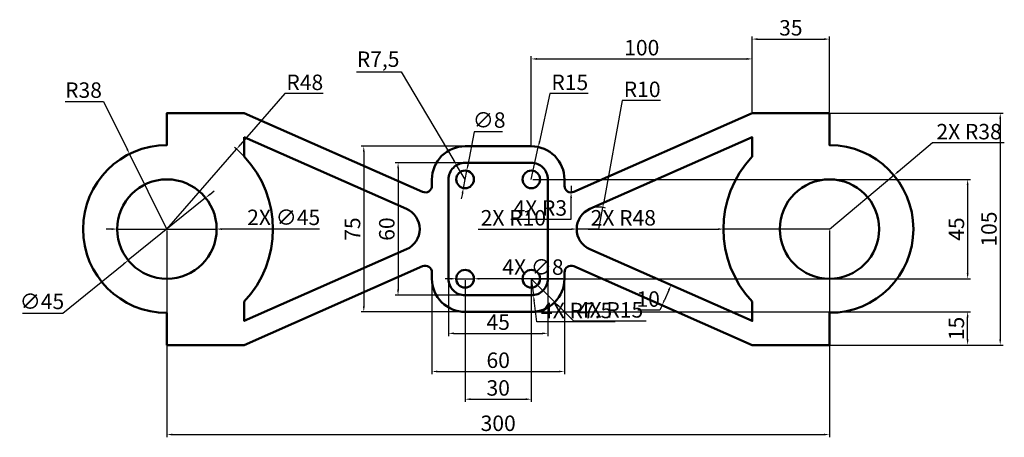
# Model space of a CAD drawing. Units: millimetres. Extents: x 172 to 618, y 203 to 392.
import ezdxf

# ---------------------------------------------------------------- set-up
doc = ezdxf.new("R2010")
doc.units = ezdxf.units.MM
doc.layers.add('M-DIMS', color=2, linetype='Continuous', lineweight=25)
doc.layers.add('M-OUTL', color=7, linetype='Continuous', lineweight=50)
doc.styles.get("Standard").update_dxf_attribs({"font": 'arial.ttf'})
doc.dimstyles.new('ISO-25', dxfattribs={"dimtxt": 7, "dimasz": 2.5, "dimexe": 1.25, "dimexo": 0.625, "dimtad": 1, "dimtoh": 1, "dimtxsty": 'Standard', "dimcen": 2.5, "dimadec": 0, "dimazin": 0, "dimtfac": 1, "dimtmove": 0, "dimatfit": 3, "dimfxl": 1, "dimarcsym": 0})

# ---------------------------------------------------------------- blocks, each defined once
blk = doc.blocks.new('*D1')
at = {"layer": 'Defpoints', "color": 0, "transparency": 16777216}
for p in [(370.22, 326.21), (374.05, 319.76)]:
    blk.add_point(p, dxfattribs=at)
at = {"layer": 'M-DIMS', "color": 0, "lineweight": -2, "transparency": 16777216}
for p, q in [((324.93, 368.48), (345.06, 368.48)), ((345.06, 368.48), (368.94, 328.35)), ((374.05, 319.76), (370.22, 326.21))]:
    blk.add_line(p, q, dxfattribs=at)
at = {"layer": 'M-DIMS', "color": 0, "transparency": 16777216}
blk.add_solid([(369.3, 328.57), (368.58, 328.14), (370.22, 326.21)], dxfattribs=at)
at = {"layer": 'M-DIMS', "color": 0, "transparency": 16777216, "insert": (334.68, 373.3), "char_height": 7, "attachment_point": 5}
blk.add_mtext('R7,5', dxfattribs=at)
blk = doc.blocks.new('*D2')
at = {"layer": 'Defpoints', "color": 0, "transparency": 16777216}
for p in [(407.22, 334.42), (404.05, 319.76)]:
    blk.add_point(p, dxfattribs=at)
at = {"layer": 'M-DIMS', "color": 0, "lineweight": -2, "transparency": 16777216}
for p, q in [((412.44, 358.61), (407.75, 336.87)), ((429.85, 358.61), (412.44, 358.61)), ((404.05, 319.76), (407.22, 334.42))]:
    blk.add_line(p, q, dxfattribs=at)
at = {"layer": 'M-DIMS', "color": 0, "transparency": 16777216}
blk.add_solid([(407.34, 336.96), (408.15, 336.78), (407.22, 334.42)], dxfattribs=at)
at = {"layer": 'M-DIMS', "color": 0, "transparency": 16777216, "insert": (421.46, 362.81), "char_height": 7, "attachment_point": 5}
blk.add_mtext('R15', dxfattribs=at)
blk = doc.blocks.new('*D3')
at = {"layer": 'Defpoints', "color": 0, "transparency": 16777216}
for p in [(389.05, 334.76), (328.19, 259.76), (389.05, 259.76)]:
    blk.add_point(p, dxfattribs=at)
at = {"layer": 'M-DIMS', "color": 0, "lineweight": -2, "transparency": 16777216}
for p, q in [((388.43, 334.76), (326.94, 334.76)), ((328.19, 332.26), (328.19, 262.26)), ((388.43, 259.76), (326.94, 259.76))]:
    blk.add_line(p, q, dxfattribs=at)
at = {"layer": 'M-DIMS', "color": 0, "transparency": 16777216}
for points in [[(327.78, 332.26), (328.61, 332.26), (328.19, 334.76)], [(327.78, 262.26), (328.61, 262.26), (328.19, 259.76)]]:
    blk.add_solid(points, dxfattribs=at)
at = {"layer": 'M-DIMS', "color": 0, "transparency": 16777216, "insert": (324.01, 297.26), "char_height": 7, "attachment_point": 5, "rotation": 90}
blk.add_mtext('75', dxfattribs=at)
blk = doc.blocks.new('*D4')
at = {"layer": 'Defpoints', "color": 0, "transparency": 16777216}
for p in [(389.05, 327.26), (343.71, 267.26), (389.05, 267.26)]:
    blk.add_point(p, dxfattribs=at)
at = {"layer": 'M-DIMS', "color": 0, "lineweight": -2, "transparency": 16777216}
for p, q in [((388.43, 327.26), (342.46, 327.26)), ((343.71, 324.76), (343.71, 269.76)), ((388.43, 267.26), (342.46, 267.26))]:
    blk.add_line(p, q, dxfattribs=at)
at = {"layer": 'M-DIMS', "color": 0, "transparency": 16777216}
for points in [[(343.3, 324.76), (344.13, 324.76), (343.71, 327.26)], [(343.3, 269.76), (344.13, 269.76), (343.71, 267.26)]]:
    blk.add_solid(points, dxfattribs=at)
at = {"layer": 'M-DIMS', "color": 0, "transparency": 16777216, "insert": (339.51, 297.26), "char_height": 7, "attachment_point": 5, "rotation": 90}
blk.add_mtext('60', dxfattribs=at)
blk = doc.blocks.new('*D5')
at = {"layer": 'Defpoints', "color": 0, "transparency": 16777216}
for p in [(270.58, 333.46), (239.05, 297.26)]:
    blk.add_point(p, dxfattribs=at)
at = {"layer": 'M-DIMS', "color": 0, "lineweight": -2, "transparency": 16777216}
for p, q in [((292.49, 358.61), (272.22, 335.34)), ((309.85, 358.61), (292.49, 358.61)), ((239.05, 297.26), (270.58, 333.46))]:
    blk.add_line(p, q, dxfattribs=at)
blk.add_arc((239.05, 297.26), 48, 43.9295, 50.4389, dxfattribs=at)
at = {"layer": 'M-DIMS', "color": 0, "transparency": 16777216}
blk.add_solid([(271.91, 335.62), (272.53, 335.07), (270.58, 333.46)], dxfattribs=at)
at = {"layer": 'M-DIMS', "color": 0, "transparency": 16777216, "insert": (301.48, 362.81), "char_height": 7, "attachment_point": 5}
blk.add_mtext('R48', dxfattribs=at)
blk = doc.blocks.new('*D6')
at = {"layer": 'Defpoints', "color": 0, "transparency": 16777216}
for p in [(222.13, 331.28), (239.05, 297.26)]:
    blk.add_point(p, dxfattribs=at)
at = {"layer": 'M-DIMS', "color": 0, "lineweight": -2, "transparency": 16777216}
for p, q in [((192.92, 355.09), (210.28, 355.09)), ((210.28, 355.09), (221.01, 333.52)), ((239.05, 297.26), (222.13, 331.28))]:
    blk.add_line(p, q, dxfattribs=at)
at = {"layer": 'M-DIMS', "color": 0, "transparency": 16777216}
blk.add_solid([(221.39, 333.71), (220.64, 333.34), (222.13, 331.28)], dxfattribs=at)
at = {"layer": 'M-DIMS', "color": 0, "transparency": 16777216, "insert": (201.29, 359.29), "char_height": 7, "attachment_point": 5}
blk.add_mtext('R38', dxfattribs=at)
blk = doc.blocks.new('*D7')
at = {"layer": 'Defpoints', "color": 0, "transparency": 16777216}
for p in [(256.56, 311.4), (221.55, 283.12)]:
    blk.add_point(p, dxfattribs=at)
at = {"layer": 'M-DIMS', "color": 0, "lineweight": -2, "transparency": 16777216}
for p, q in [((258.5, 312.97), (260.45, 314.54)), ((256.56, 311.4), (221.55, 283.12)), ((191.94, 259.2), (219.61, 281.55)), ((173.61, 259.2), (191.94, 259.2))]:
    blk.add_line(p, q, dxfattribs=at)
at = {"layer": 'M-DIMS', "color": 0, "transparency": 16777216}
for points in [[(258.24, 313.29), (258.76, 312.65), (256.56, 311.4)], [(219.34, 281.88), (219.87, 281.23), (221.55, 283.12)]]:
    blk.add_solid(points, dxfattribs=at)
at = {"layer": 'M-DIMS', "color": 0, "transparency": 16777216, "insert": (182.46, 263.6), "char_height": 7, "attachment_point": 5}
blk.add_mtext('∅45', dxfattribs=at)
blk = doc.blocks.new('*D8')
at = {"layer": 'Defpoints', "color": 0, "transparency": 16777216}
for p in [(239.05, 297.26), (539.05, 297.26), (539.05, 204.21)]:
    blk.add_point(p, dxfattribs=at)
at = {"layer": 'M-DIMS', "color": 0, "lineweight": -2, "transparency": 16777216}
for p, q in [((239.05, 296.64), (239.05, 202.96)), ((539.05, 296.64), (539.05, 202.96)), ((241.55, 204.21), (536.55, 204.21))]:
    blk.add_line(p, q, dxfattribs=at)
at = {"layer": 'M-DIMS', "color": 0, "transparency": 16777216}
for points in [[(241.55, 204.62), (241.55, 203.79), (239.05, 204.21)], [(536.55, 204.62), (536.55, 203.79), (539.05, 204.21)]]:
    blk.add_solid(points, dxfattribs=at)
at = {"layer": 'M-DIMS', "color": 0, "transparency": 16777216, "insert": (389.05, 208.41), "char_height": 7, "attachment_point": 5}
blk.add_mtext('300', dxfattribs=at)
blk = doc.blocks.new('*D9')
at = {"layer": 'Defpoints', "color": 0, "transparency": 16777216}
for p in [(359.05, 274.76), (419.05, 274.76), (419.05, 232.76)]:
    blk.add_point(p, dxfattribs=at)
at = {"layer": 'M-DIMS', "color": 0, "lineweight": -2, "transparency": 16777216}
for p, q in [((359.05, 274.14), (359.05, 231.51)), ((419.05, 274.14), (419.05, 231.51)), ((361.55, 232.76), (416.55, 232.76))]:
    blk.add_line(p, q, dxfattribs=at)
at = {"layer": 'M-DIMS', "color": 0, "transparency": 16777216}
for points in [[(361.55, 233.18), (361.55, 232.35), (359.05, 232.76)], [(416.55, 233.18), (416.55, 232.35), (419.05, 232.76)]]:
    blk.add_solid(points, dxfattribs=at)
at = {"layer": 'M-DIMS', "color": 0, "transparency": 16777216, "insert": (389.05, 236.96), "char_height": 7, "attachment_point": 5}
blk.add_mtext('60', dxfattribs=at)
blk = doc.blocks.new('*D10')
at = {"layer": 'Defpoints', "color": 0, "transparency": 16777216}
for p in [(366.55, 288.46), (411.55, 288.46), (411.55, 250.04)]:
    blk.add_point(p, dxfattribs=at)
at = {"layer": 'M-DIMS', "color": 0, "lineweight": -2, "transparency": 16777216}
for p, q in [((366.55, 287.84), (366.55, 248.79)), ((411.55, 287.84), (411.55, 248.79)), ((369.05, 250.04), (409.05, 250.04))]:
    blk.add_line(p, q, dxfattribs=at)
at = {"layer": 'M-DIMS', "color": 0, "transparency": 16777216}
for points in [[(369.05, 250.45), (369.05, 249.62), (366.55, 250.04)], [(409.05, 250.45), (409.05, 249.62), (411.55, 250.04)]]:
    blk.add_solid(points, dxfattribs=at)
at = {"layer": 'M-DIMS', "color": 0, "transparency": 16777216, "insert": (389.05, 254.22), "char_height": 7, "attachment_point": 5}
blk.add_mtext('45', dxfattribs=at)
blk = doc.blocks.new('*D11')
at = {"layer": 'Defpoints', "color": 0, "transparency": 16777216}
for p in [(374.81, 323.69), (373.3, 315.83)]:
    blk.add_point(p, dxfattribs=at)
at = {"layer": 'M-DIMS', "color": 0, "lineweight": -2, "transparency": 16777216}
for p, q in [((378.22, 341.34), (375.29, 326.14)), ((391.06, 341.34), (378.22, 341.34)), ((373.3, 315.83), (374.81, 323.69)), ((372.82, 313.38), (372.35, 310.92))]:
    blk.add_line(p, q, dxfattribs=at)
at = {"layer": 'M-DIMS', "color": 0, "transparency": 16777216}
for points in [[(374.88, 326.22), (375.7, 326.06), (374.81, 323.69)], [(372.41, 313.46), (373.23, 313.3), (373.3, 315.83)]]:
    blk.add_solid(points, dxfattribs=at)
at = {"layer": 'M-DIMS', "color": 0, "transparency": 16777216, "insert": (384.95, 345.73), "char_height": 7, "attachment_point": 5}
blk.add_mtext('∅8', dxfattribs=at)
blk = doc.blocks.new('*D12')
at = {"layer": 'Defpoints', "color": 0, "transparency": 16777216}
for p in [(436.4, 307.1), (434.6, 297.26)]:
    blk.add_point(p, dxfattribs=at)
at = {"layer": 'M-DIMS', "color": 0, "lineweight": -2, "transparency": 16777216}
for p, q in [((445.25, 355.44), (436.85, 309.56)), ((462.58, 355.44), (445.25, 355.44)), ((434.6, 297.26), (436.4, 307.1))]:
    blk.add_line(p, q, dxfattribs=at)
blk.add_arc((434.6, 297.26), 10, 72.4639, 110.225, dxfattribs=at)
at = {"layer": 'M-DIMS', "color": 0, "transparency": 16777216}
blk.add_solid([(436.44, 309.63), (437.26, 309.48), (436.4, 307.1)], dxfattribs=at)
at = {"layer": 'M-DIMS', "color": 0, "transparency": 16777216, "insert": (454.23, 359.64), "char_height": 7, "attachment_point": 5}
blk.add_mtext('R10', dxfattribs=at)
blk = doc.blocks.new('*D13')
at = {"layer": 'Defpoints', "color": 0, "transparency": 16777216}
for p in [(539.05, 383.29), (504.05, 349.76), (539.05, 349.76)]:
    blk.add_point(p, dxfattribs=at)
at = {"layer": 'M-DIMS', "color": 0, "lineweight": -2, "transparency": 16777216}
for p, q in [((504.05, 350.39), (504.05, 384.54)), ((539.05, 350.39), (539.05, 384.54)), ((506.55, 383.29), (536.55, 383.29))]:
    blk.add_line(p, q, dxfattribs=at)
at = {"layer": 'M-DIMS', "color": 0, "transparency": 16777216}
for points in [[(506.55, 383.71), (506.55, 382.87), (504.05, 383.29)], [(536.55, 383.71), (536.55, 382.87), (539.05, 383.29)]]:
    blk.add_solid(points, dxfattribs=at)
at = {"layer": 'M-DIMS', "color": 0, "transparency": 16777216, "insert": (521.55, 387.49), "char_height": 7, "attachment_point": 5}
blk.add_mtext('35', dxfattribs=at)
blk = doc.blocks.new('*D14')
at = {"layer": 'Defpoints', "color": 0, "transparency": 16777216}
for p in [(521.55, 349.76), (521.55, 244.76), (616.37, 244.76)]:
    blk.add_point(p, dxfattribs=at)
at = {"layer": 'M-DIMS', "color": 0, "lineweight": -2, "transparency": 16777216}
for p, q in [((522.18, 349.76), (617.62, 349.76)), ((616.37, 347.26), (616.37, 247.26)), ((522.18, 244.76), (617.62, 244.76))]:
    blk.add_line(p, q, dxfattribs=at)
at = {"layer": 'M-DIMS', "color": 0, "transparency": 16777216}
for points in [[(615.95, 347.26), (616.78, 347.26), (616.37, 349.76)], [(615.95, 247.26), (616.78, 247.26), (616.37, 244.76)]]:
    blk.add_solid(points, dxfattribs=at)
at = {"layer": 'M-DIMS', "color": 0, "transparency": 16777216, "insert": (612.17, 297.26), "char_height": 7, "attachment_point": 5, "rotation": 90}
blk.add_mtext('105', dxfattribs=at)
blk = doc.blocks.new('*D15')
at = {"layer": 'Defpoints', "color": 0, "transparency": 16777216}
for p in [(467.31, 271.9), (463.27, 262.75), (463.27, 262.75)]:
    blk.add_point(p, dxfattribs=at)
at = {"layer": 'M-DIMS', "color": 0, "lineweight": -2, "transparency": 16777216}
for p, q in [((466.74, 272.15), (466.17, 272.41)), ((466.3, 269.61), (464.28, 265.04)), ((462.7, 263), (462.13, 263.26)), ((462.26, 260.47), (452.3, 260.47)), ((463.27, 262.75), (462.26, 260.47))]:
    blk.add_line(p, q, dxfattribs=at)
at = {"layer": 'M-DIMS', "color": 0, "transparency": 16777216}
for points in [[(465.92, 269.78), (466.68, 269.45), (467.31, 271.9)], [(463.9, 265.21), (464.66, 264.87), (463.27, 262.75)]]:
    blk.add_solid(points, dxfattribs=at)
at = {"layer": 'M-DIMS', "color": 0, "transparency": 16777216, "insert": (456.97, 264.66), "char_height": 7, "attachment_point": 5}
blk.add_mtext('10', dxfattribs=at)
blk = doc.blocks.new('*D16')
at = {"layer": 'Defpoints', "color": 0, "transparency": 16777216}
for p in [(504.05, 374.31), (504.05, 349.76), (404.05, 334.76)]:
    blk.add_point(p, dxfattribs=at)
at = {"layer": 'M-DIMS', "color": 0, "lineweight": -2, "transparency": 16777216}
for p, q in [((404.05, 335.39), (404.05, 375.56)), ((504.05, 350.39), (504.05, 375.56)), ((406.55, 374.31), (501.55, 374.31))]:
    blk.add_line(p, q, dxfattribs=at)
at = {"layer": 'M-DIMS', "color": 0, "transparency": 16777216}
for points in [[(406.55, 374.73), (406.55, 373.89), (404.05, 374.31)], [(501.55, 374.73), (501.55, 373.89), (504.05, 374.31)]]:
    blk.add_solid(points, dxfattribs=at)
at = {"layer": 'M-DIMS', "color": 0, "transparency": 16777216, "insert": (454.05, 378.51), "char_height": 7, "attachment_point": 5}
blk.add_mtext('100', dxfattribs=at)
blk = doc.blocks.new('*D17')
at = {"layer": 'Defpoints', "color": 0, "transparency": 16777216}
for p in [(404.05, 259.76), (601.6, 259.76), (504.05, 244.76)]:
    blk.add_point(p, dxfattribs=at)
at = {"layer": 'M-DIMS', "color": 0, "lineweight": -2, "transparency": 16777216}
for p, q in [((404.68, 259.76), (602.85, 259.76)), ((601.6, 247.26), (601.6, 257.26)), ((504.68, 244.76), (602.85, 244.76))]:
    blk.add_line(p, q, dxfattribs=at)
at = {"layer": 'M-DIMS', "color": 0, "transparency": 16777216}
for points in [[(601.19, 257.26), (602.02, 257.26), (601.6, 259.76)], [(601.19, 247.26), (602.02, 247.26), (601.6, 244.76)]]:
    blk.add_solid(points, dxfattribs=at)
at = {"layer": 'M-DIMS', "color": 0, "transparency": 16777216, "insert": (597.4, 252.26), "char_height": 7, "attachment_point": 5, "rotation": 90}
blk.add_mtext('15', dxfattribs=at)
blk = doc.blocks.new('*D18')
at = {"layer": 'Defpoints', "color": 0, "transparency": 16777216}
for p in [(374.05, 274.76), (404.05, 274.76), (404.05, 220.21)]:
    blk.add_point(p, dxfattribs=at)
at = {"layer": 'M-DIMS', "color": 0, "lineweight": -2, "transparency": 16777216}
for p, q in [((374.05, 274.14), (374.05, 218.96)), ((404.05, 274.14), (404.05, 218.96)), ((376.55, 220.21), (401.55, 220.21))]:
    blk.add_line(p, q, dxfattribs=at)
at = {"layer": 'M-DIMS', "color": 0, "transparency": 16777216}
for points in [[(376.55, 220.63), (376.55, 219.79), (374.05, 220.21)], [(401.55, 220.63), (401.55, 219.79), (404.05, 220.21)]]:
    blk.add_solid(points, dxfattribs=at)
at = {"layer": 'M-DIMS', "color": 0, "transparency": 16777216, "insert": (389.05, 224.41), "char_height": 7, "attachment_point": 5}
blk.add_mtext('30', dxfattribs=at)
blk = doc.blocks.new('*D19')
at = {"layer": 'Defpoints', "color": 0, "transparency": 16777216}
for p in [(404.05, 319.76), (404.05, 274.76), (601.6, 274.76)]:
    blk.add_point(p, dxfattribs=at)
at = {"layer": 'M-DIMS', "color": 0, "lineweight": -2, "transparency": 16777216}
for p, q in [((404.68, 319.76), (602.85, 319.76)), ((601.6, 317.26), (601.6, 277.26)), ((404.68, 274.76), (602.85, 274.76))]:
    blk.add_line(p, q, dxfattribs=at)
at = {"layer": 'M-DIMS', "color": 0, "transparency": 16777216}
for points in [[(601.19, 317.26), (602.02, 317.26), (601.6, 319.76)], [(601.19, 277.26), (602.02, 277.26), (601.6, 274.76)]]:
    blk.add_solid(points, dxfattribs=at)
at = {"layer": 'M-DIMS', "color": 0, "transparency": 16777216, "insert": (597.42, 297.26), "char_height": 7, "attachment_point": 5, "rotation": 90}
blk.add_mtext('45', dxfattribs=at)
blk = doc.blocks.new('*D20')
at = {"layer": 'Defpoints', "color": 0, "transparency": 16777216}
for p in [(568.2, 321.65), (539.05, 297.26)]:
    blk.add_point(p, dxfattribs=at)
at = {"layer": 'M-DIMS', "color": 0, "lineweight": -2, "transparency": 16777216}
for p, q in [((585.68, 336.28), (570.11, 323.25)), ((618.21, 336.28), (585.68, 336.28)), ((539.05, 297.26), (568.2, 321.65))]:
    blk.add_line(p, q, dxfattribs=at)
at = {"layer": 'M-DIMS', "color": 0, "transparency": 16777216}
blk.add_solid([(569.85, 323.57), (570.38, 322.93), (568.2, 321.65)], dxfattribs=at)
at = {"layer": 'M-DIMS', "color": 0, "transparency": 16777216, "insert": (602.26, 340.48), "char_height": 7, "attachment_point": 5}
blk.add_mtext('2X R38', dxfattribs=at)
blk = doc.blocks.new('*D21')
at = {"layer": 'Defpoints', "color": 0, "transparency": 16777216}
for p in [(216.55, 297.26), (261.55, 297.26)]:
    blk.add_point(p, dxfattribs=at)
at = {"layer": 'M-DIMS', "color": 0, "lineweight": -2, "transparency": 16777216}
for p, q in [((214.05, 297.26), (211.55, 297.26)), ((216.55, 297.26), (261.55, 297.26)), ((275.05, 297.26), (264.05, 297.26)), ((308.16, 297.26), (275.05, 297.26))]:
    blk.add_line(p, q, dxfattribs=at)
at = {"layer": 'M-DIMS', "color": 0, "transparency": 16777216}
for points in [[(214.05, 297.68), (214.05, 296.85), (216.55, 297.26)], [(264.05, 297.68), (264.05, 296.84), (261.55, 297.26)]]:
    blk.add_solid(points, dxfattribs=at)
at = {"layer": 'M-DIMS', "color": 0, "transparency": 16777216, "insert": (291.92, 301.66), "char_height": 7, "attachment_point": 5}
blk.add_mtext('2X ∅45', dxfattribs=at)
blk = doc.blocks.new('*D22')
at = {"layer": 'Defpoints', "color": 0, "transparency": 16777216}
for p in [(491.05, 297.26), (539.05, 297.26)]:
    blk.add_point(p, dxfattribs=at)
at = {"layer": 'M-DIMS', "color": 0, "lineweight": -2, "transparency": 16777216}
for p, q in [((429.73, 297.26), (462.25, 297.26)), ((462.25, 297.26), (488.55, 297.26)), ((539.05, 297.26), (491.05, 297.26))]:
    blk.add_line(p, q, dxfattribs=at)
at = {"layer": 'M-DIMS', "color": 0, "transparency": 16777216}
blk.add_solid([(488.55, 297.68), (488.55, 296.84), (491.05, 297.26)], dxfattribs=at)
at = {"layer": 'M-DIMS', "color": 0, "transparency": 16777216, "insert": (445.68, 301.46), "char_height": 7, "attachment_point": 5}
blk.add_mtext('2X R48', dxfattribs=at)
blk = doc.blocks.new('*D23')
at = {"layer": 'Defpoints', "color": 0, "transparency": 16777216}
for p in [(424.6, 297.26), (434.6, 297.26)]:
    blk.add_point(p, dxfattribs=at)
at = {"layer": 'M-DIMS', "color": 0, "lineweight": -2, "transparency": 16777216}
for p, q in [((379.97, 297.26), (412.45, 297.26)), ((412.45, 297.26), (422.1, 297.26)), ((434.6, 297.26), (424.6, 297.26))]:
    blk.add_line(p, q, dxfattribs=at)
at = {"layer": 'M-DIMS', "color": 0, "transparency": 16777216}
blk.add_solid([(422.1, 297.68), (422.1, 296.84), (424.6, 297.26)], dxfattribs=at)
at = {"layer": 'M-DIMS', "color": 0, "transparency": 16777216, "insert": (395.9, 301.46), "char_height": 7, "attachment_point": 5}
blk.add_mtext('2X R10', dxfattribs=at)
blk = doc.blocks.new('*D24')
at = {"layer": 'Defpoints', "color": 0, "transparency": 16777216}
for p in [(404.05, 274.76), (414.66, 264.15)]:
    blk.add_point(p, dxfattribs=at)
at = {"layer": 'M-DIMS', "color": 0, "lineweight": -2, "transparency": 16777216}
for p, q in [((404.05, 274.76), (414.66, 264.15)), ((423.25, 255.56), (416.43, 262.39)), ((455.98, 255.56), (423.25, 255.56))]:
    blk.add_line(p, q, dxfattribs=at)
at = {"layer": 'M-DIMS', "color": 0, "transparency": 16777216}
blk.add_solid([(416.72, 262.68), (416.13, 262.09), (414.66, 264.15)], dxfattribs=at)
at = {"layer": 'M-DIMS', "color": 0, "transparency": 16777216, "insert": (439.93, 259.76), "char_height": 7, "attachment_point": 5}
blk.add_mtext('4X R15', dxfattribs=at)
blk = doc.blocks.new('*D25')
at = {"layer": 'Defpoints', "color": 0, "transparency": 16777216}
for p in [(404.05, 274.76), (405, 267.32)]:
    blk.add_point(p, dxfattribs=at)
at = {"layer": 'M-DIMS', "color": 0, "lineweight": -2, "transparency": 16777216}
for p, q in [((404.05, 274.76), (405, 267.32)), ((406.53, 255.3), (405.32, 264.84)), ((441.98, 255.3), (406.53, 255.3))]:
    blk.add_line(p, q, dxfattribs=at)
at = {"layer": 'M-DIMS', "color": 0, "transparency": 16777216}
blk.add_solid([(405.73, 264.89), (404.9, 264.79), (405, 267.32)], dxfattribs=at)
at = {"layer": 'M-DIMS', "color": 0, "transparency": 16777216, "insert": (424.57, 259.48), "char_height": 7, "attachment_point": 5}
blk.add_mtext('4X R7.5', dxfattribs=at)
blk = doc.blocks.new('*D26')
at = {"layer": 'Defpoints', "color": 0, "transparency": 16777216}
for p in [(370.05, 274.76), (378.05, 274.76)]:
    blk.add_point(p, dxfattribs=at)
at = {"layer": 'M-DIMS', "color": 0, "lineweight": -2, "transparency": 16777216}
for p, q in [((367.55, 274.76), (365.05, 274.76)), ((370.05, 274.76), (378.05, 274.76)), ((390.59, 274.76), (380.55, 274.76)), ((418.39, 274.76), (390.59, 274.76))]:
    blk.add_line(p, q, dxfattribs=at)
at = {"layer": 'M-DIMS', "color": 0, "transparency": 16777216}
for points in [[(367.55, 275.18), (367.55, 274.35), (370.05, 274.76)], [(380.55, 275.18), (380.55, 274.34), (378.05, 274.76)]]:
    blk.add_solid(points, dxfattribs=at)
at = {"layer": 'M-DIMS', "color": 0, "transparency": 16777216, "insert": (404.8, 279.15), "char_height": 7, "attachment_point": 5}
blk.add_mtext('4X ∅8', dxfattribs=at)
blk = doc.blocks.new('*D27')
at = {"layer": 'Defpoints', "color": 0, "transparency": 16777216}
for p in [(422.05, 316.86), (422.05, 313.86)]:
    blk.add_point(p, dxfattribs=at)
at = {"layer": 'M-DIMS', "color": 0, "lineweight": -2, "transparency": 16777216}
for p, q in [((422.05, 316.86), (422.05, 313.86)), ((422.03, 301.71), (422.05, 311.36)), ((394.8, 301.71), (422.03, 301.71))]:
    blk.add_line(p, q, dxfattribs=at)
at = {"layer": 'M-DIMS', "color": 0, "transparency": 16777216}
blk.add_solid([(421.63, 311.36), (422.46, 311.36), (422.05, 313.86)], dxfattribs=at)
at = {"layer": 'M-DIMS', "color": 0, "transparency": 16777216, "insert": (408.1, 305.91), "char_height": 7, "attachment_point": 5}
blk.add_mtext('4X R3', dxfattribs=at)

msp = doc.modelspace()

# ---------------------------------------------------------------- linework, layer by layer
at = {"layer": 'M-OUTL'}
for points in [[(419.054, 274.761), (419.054, 277.659, -0.5418599), (423.265, 280.404), (504.054, 244.761), (539.054, 244.761), (539.054, 259.261, 1), (539.054, 335.261), (539.054, 349.761), (504.054, 349.761), (423.265, 314.119, -0.5418599), (419.054, 316.864), (419.054, 319.761, 0.4142136), (404.054, 334.761), (374.054, 334.761, 0.4142136), (359.054, 319.761), (359.054, 316.864, -0.5418599), (354.843, 314.119), (274.054, 349.761), (239.054, 349.761), (239.054, 335.261, 1), (239.054, 259.261), (239.054, 244.761), (274.054, 244.761), (354.843, 280.404, -0.5418599), (359.054, 277.659), (359.054, 274.761, 0.4142136), (374.054, 259.761), (404.054, 259.761, 0.4142136)], [(274.054, 338.831), (274.054, 330.11, -0.3957607), (274.054, 264.413), (274.054, 255.691), (347.541, 288.112, 0.6518179), (347.541, 306.411)], [(430.567, 288.112, -0.6518179), (430.567, 306.411), (504.054, 338.831), (504.054, 330.11, 0.3957607), (504.054, 264.413), (504.054, 255.691)], [(404.054, 327.261), (374.054, 327.261, 0.4142136), (366.554, 319.761), (366.554, 274.761, 0.4142136), (374.054, 267.261), (404.054, 267.261, 0.4142136), (411.554, 274.761), (411.554, 319.761, 0.4142136)]]:
    msp.add_lwpolyline(points, format="xyb", close=True, dxfattribs=at)
for centre, radius in [((374.054, 319.761), 4), ((404.054, 319.761), 4), ((239.054, 297.261), 22.5), ((539.054, 297.261), 22.5), ((374.054, 274.761), 4), ((404.054, 274.761), 4)]:
    msp.add_circle(centre, radius, dxfattribs=at)

# ---------------------------------------------------------------- dimensions: what is measured, and where the dimension line sits
at = {"layer": 'M-DIMS'}
for base, p1, p2, override, picture, middle in [((539.054, 383.291), (504.054, 349.761), (539.054, 349.761), {"dimclrd": 0, "dimclre": 0, "dimclrt": 0}, '*D13', (521.554, 387.492)), ((504.054, 374.311), (404.054, 334.761), (504.054, 349.761), {"dimdec": 0, "dimlfac": 1, "dimrnd": 0, "dimzin": 0, "dimdsep": 46, "dimlunit": 2}, '*D16', (454.054, 378.51)), ((539.054, 204.208), (239.054, 297.261), (539.054, 297.261), {"dimclrd": 0, "dimclre": 0, "dimclrt": 0}, '*D8', (389.054, 208.41)), ((411.554, 250.036), (366.554, 288.461), (411.554, 288.461), {"dimclrd": 0, "dimclre": 0, "dimclrt": 0}, '*D10', (389.054, 254.221)), ((419.054, 232.763), (359.054, 274.761), (419.054, 274.761), {"dimclrd": 0, "dimclre": 0, "dimclrt": 0}, '*D9', (389.054, 236.962)), ((404.054, 220.211), (374.054, 274.761), (404.054, 274.761), {"dimdec": 0, "dimlfac": 1, "dimrnd": 0, "dimzin": 0, "dimdsep": 46, "dimlunit": 2}, '*D18', (389.054, 224.413))]:
    dim = msp.add_linear_dim(base=base, p1=p1, p2=p2, dimstyle='ISO-25', override=override, dxfattribs=at)
    dim.commit()
    dim.dimension.update_dxf_attribs({"geometry": picture, "text_midpoint": middle})
for center, mpoint, picture, middle in [((374.054, 319.761), (370.218, 326.206), '*D1', (334.683, 368.485)), ((239.054, 297.261), (270.578, 333.458), '*D5', (301.482, 358.614)), ((404.054, 319.761), (407.22, 334.424), '*D2', (421.457, 358.614)), ((239.054, 297.261), (222.126, 331.283), '*D6', (201.287, 355.089)), ((434.603, 297.261), (436.404, 307.098), '*D12', (454.23, 355.441))]:
    dim = msp.add_radius_dim(center=center, mpoint=mpoint, dimstyle='ISO-25', override={"dimclrd": 0, "dimclre": 0, "dimclrt": 0}, dxfattribs=at)
    dim.commit()
    dim.dimension.update_dxf_attribs({"geometry": picture, "text_midpoint": middle, "dimtype": 164})
for p1, p2, picture, middle in [((373.296, 315.834), (374.812, 323.689), '*D11', (384.954, 341.34)), ((256.557, 311.4), (221.551, 283.123), '*D7', (182.463, 259.202))]:
    dim = msp.add_diameter_dim_2p(p1=p1, p2=p2, dimstyle='ISO-25', override={"dimclrd": 0, "dimclre": 0, "dimclrt": 0}, dxfattribs=at)
    dim.commit()
    dim.dimension.update_dxf_attribs({"geometry": picture, "text_midpoint": middle, "dimtype": 163})
for base, p1, p2, override, picture, middle in [((616.367, 244.761), (521.554, 349.761), (521.554, 244.761), {"dimclrd": 0, "dimclre": 0, "dimclrt": 0}, '*D14', (612.168, 297.261)), ((328.195, 259.761), (389.054, 334.761), (389.054, 259.761), {"dimclrd": 0, "dimclre": 0, "dimclrt": 0}, '*D3', (324.01, 297.261)), ((343.713, 267.261), (389.054, 327.261), (389.054, 267.261), {"dimclrd": 0, "dimclre": 0, "dimclrt": 0}, '*D4', (339.514, 297.261)), ((601.604, 274.761), (404.054, 319.761), (404.054, 274.761), {"dimdec": 0, "dimlfac": 1, "dimrnd": 0, "dimzin": 0, "dimdsep": 46, "dimlunit": 2}, '*D19', (597.419, 297.261)), ((601.604, 259.761), (504.054, 244.761), (404.054, 259.761), {"dimdec": 0, "dimlfac": 1, "dimrnd": 0, "dimzin": 0, "dimdsep": 46, "dimlunit": 2}, '*D17', (597.405, 252.261))]:
    dim = msp.add_linear_dim(base=base, p1=p1, p2=p2, angle=90, dimstyle='ISO-25', override=override, dxfattribs=at)
    dim.commit()
    dim.dimension.update_dxf_attribs({"geometry": picture, "text_midpoint": middle})
for mpoint, picture, middle in [((568.197, 321.647), '*D20', (602.258, 336.279)), ((491.054, 297.261), '*D22', (462.254, 297.261))]:
    dim = msp.add_radius_dim(center=(539.054, 297.261), mpoint=mpoint, text='2X <>', dimstyle='ISO-25', override={"dimdec": 0, "dimlfac": 1, "dimrnd": 0, "dimzin": 0, "dimdsep": 46, "dimlunit": 2}, dxfattribs=at)
    dim.commit()
    dim.dimension.update_dxf_attribs({"geometry": picture, "text_midpoint": middle, "dimtype": 164})
for center, mpoint, text, override, picture, middle in [((422.054, 316.864), (422.05, 313.864), '4X <>', {"dimdec": 0, "dimlfac": 1, "dimrnd": 0, "dimzin": 0, "dimdsep": 46, "dimlunit": 2}, '*D27', (408.104, 305.913)), ((434.603, 297.261), (424.603, 297.261), '2X <>', {"dimdec": 0, "dimlfac": 1, "dimrnd": 0, "dimzin": 0, "dimdsep": 46, "dimlunit": 2}, '*D23', (395.898, 301.459)), ((404.054, 274.761), (414.66, 264.155), '4X <>', {"dimdec": 0, "dimlfac": 1, "dimrnd": 0, "dimzin": 0, "dimdsep": 46, "dimlunit": 2}, '*D24', (439.926, 259.764)), ((404.054, 274.761), (405.001, 267.321), '4X <>', {"dimdec": 1, "dimlfac": 1, "dimrnd": 0, "dimzin": 0, "dimdsep": 46, "dimlunit": 2}, '*D25', (424.566, 259.484))]:
    dim = msp.add_radius_dim(center=center, mpoint=mpoint, text=text, dimstyle='ISO-25', override=override, dxfattribs=at)
    dim.commit()
    dim.dimension.update_dxf_attribs({"geometry": picture, "text_midpoint": middle})
for p1, p2, text, picture, middle in [((216.554, 297.262), (261.554, 297.261), '2X <>', '*D21', (275.054, 297.261)), ((370.054, 274.762), (378.054, 274.761), '4X <>', '*D26', (390.593, 274.76))]:
    dim = msp.add_diameter_dim_2p(p1=p1, p2=p2, text=text, dimstyle='ISO-25', override={"dimdec": 0, "dimlfac": 1, "dimrnd": 0, "dimzin": 0, "dimdsep": 46, "dimlunit": 2}, dxfattribs=at)
    dim.commit()
    dim.dimension.update_dxf_attribs({"geometry": picture, "text_midpoint": middle, "dimtype": 163})
dim = msp.add_aligned_dim(p1=(467.31, 271.902), p2=(463.274, 262.753), distance=0, dimstyle='ISO-25', override={"dimclrd": 0, "dimclre": 0, "dimclrt": 0}, dxfattribs=at)
dim.commit()
dim.dimension.update_dxf_attribs({"geometry": '*D15', "text_midpoint": (456.967, 264.664)})

doc.saveas('drawing.dxf')
